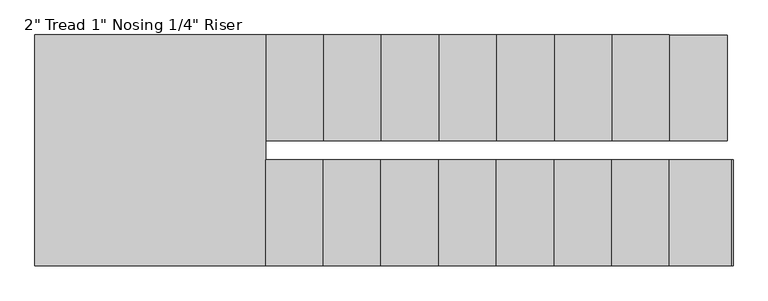
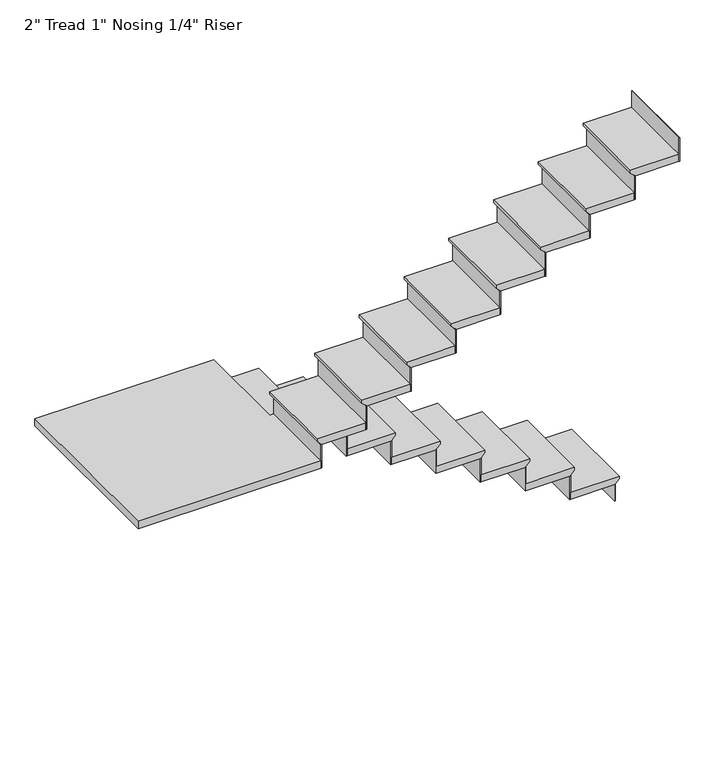
"""IFC4 building model written with IfcOpenShell, lengths in millimetres: stair flight geometry."""

from ifc_helpers import new_model, si_unit, origin, place, context, project, spatial, faceted_brep, source, transform, mapped, element, save


def stair_flight_6b4fcaec(model_context):
    return source(origin(), model_context, "Body", "Brep", [
        faceted_brep([(-1805.9198569, -5306.3933037, 12951.8833333), (-1805.9198569, -5306.3933037, 12970.9333333), (-1805.9198569, -5865.1933037, 12970.9333333), (-1805.9198569, -5865.1933037, 12951.8833333), (-1831.3198569, -5306.3933037, 12926.4833333), (-1831.3198569, -5865.1933037, 12926.4833333), (-2136.1198569, -5306.3933037, 12970.9333333), (-2136.1198569, -5865.1933037, 12970.9333333), (-1831.3198569, -5865.1933037, 12920.1333333), (-2136.1198569, -5865.1933037, 12920.1333333), (-2136.1198569, -5306.3933037, 12920.1333333), (-1831.3198569, -5306.3933037, 12920.1333333)], [[[0, 1, 2, 3]], [[4, 0, 3, 5]], [[2, 1, 6, 7]], [[8, 9, 10, 11]], [[2, 7, 9, 8, 5, 3]], [[8, 11, 4, 5]], [[6, 1, 0, 4, 11, 10]], [[7, 6, 10, 9]]]),
        faceted_brep([(-1831.3198569, -5306.3933037, 12920.1333333), (-1831.3198569, -5306.3933037, 12801.6), (-1837.6698569, -5306.3933037, 12801.6), (-1837.6698569, -5306.3933037, 12920.1333333), (-1831.3198569, -5865.1933037, 12920.1333333), (-1837.6698569, -5865.1933037, 12920.1333333), (-1837.6698569, -5865.1933037, 12801.6), (-1831.3198569, -5865.1933037, 12801.6)], [[[0, 1, 2, 3]], [[4, 5, 6, 7]], [[1, 0, 4, 7]], [[2, 1, 7, 6]], [[3, 2, 6, 5]], [[0, 3, 5, 4]]]),
        faceted_brep([(-2136.1198569, -5306.3933037, 13089.4666667), (-2136.1198569, -5306.3933037, 12920.1333333), (-2142.4698569, -5306.3933037, 12920.1333333), (-2142.4698569, -5306.3933037, 13089.4666667), (-2136.1198569, -5865.1933037, 13089.4666667), (-2142.4698569, -5865.1933037, 13089.4666667), (-2142.4698569, -5865.1933037, 12920.1333333), (-2136.1198569, -5865.1933037, 12920.1333333)], [[[0, 1, 2, 3]], [[4, 5, 6, 7]], [[1, 0, 4, 7]], [[2, 1, 7, 6]], [[3, 2, 6, 5]], [[0, 3, 5, 4]]]),
        faceted_brep([(-2110.7198569, -5865.1933037, 13140.2666667), (-2110.7198569, -5306.3933037, 13140.2666667), (-2440.9198569, -5306.3933037, 13140.2666667), (-2440.9198569, -5865.1933037, 13140.2666667), (-2136.1198569, -5865.1933037, 13089.4666667), (-2440.9198569, -5865.1933037, 13089.4666667), (-2440.9198569, -5306.3933037, 13089.4666667), (-2136.1198569, -5306.3933037, 13089.4666667), (-2136.1198569, -5865.1933037, 13095.8166667), (-2110.7198569, -5865.1933037, 13121.2166667), (-2136.1198569, -5306.3933037, 13095.8166667), (-2110.7198569, -5306.3933037, 13121.2166667)], [[[0, 1, 2, 3]], [[4, 5, 6, 7]], [[0, 3, 5, 4, 8, 9]], [[4, 7, 10, 8]], [[2, 1, 11, 10, 7, 6]], [[3, 2, 6, 5]], [[11, 1, 0, 9]], [[10, 11, 9, 8]]]),
        faceted_brep([(-2440.9198569, -5306.3933037, 13258.8), (-2440.9198569, -5306.3933037, 13089.4666667), (-2447.2698569, -5306.3933037, 13089.4666667), (-2447.2698569, -5306.3933037, 13258.8), (-2440.9198569, -5865.1933037, 13258.8), (-2447.2698569, -5865.1933037, 13258.8), (-2447.2698569, -5865.1933037, 13089.4666667), (-2440.9198569, -5865.1933037, 13089.4666667)], [[[0, 1, 2, 3]], [[4, 5, 6, 7]], [[1, 0, 4, 7]], [[2, 1, 7, 6]], [[3, 2, 6, 5]], [[0, 3, 5, 4]]]),
        faceted_brep([(-2415.5198569, -5865.1933037, 13309.6), (-2415.5198569, -5306.3933037, 13309.6), (-2745.7198569, -5306.3933037, 13309.6), (-2745.7198569, -5865.1933037, 13309.6), (-2440.9198569, -5865.1933037, 13258.8), (-2745.7198569, -5865.1933037, 13258.8), (-2745.7198569, -5306.3933037, 13258.8), (-2440.9198569, -5306.3933037, 13258.8), (-2440.9198569, -5865.1933037, 13265.15), (-2415.5198569, -5865.1933037, 13290.55), (-2440.9198569, -5306.3933037, 13265.15), (-2415.5198569, -5306.3933037, 13290.55)], [[[0, 1, 2, 3]], [[4, 5, 6, 7]], [[0, 3, 5, 4, 8, 9]], [[4, 7, 10, 8]], [[2, 1, 11, 10, 7, 6]], [[3, 2, 6, 5]], [[11, 1, 0, 9]], [[10, 11, 9, 8]]]),
        faceted_brep([(-2745.7198569, -5306.3933037, 13428.1333333), (-2745.7198569, -5306.3933037, 13258.8), (-2752.0698569, -5306.3933037, 13258.8), (-2752.0698569, -5306.3933037, 13428.1333333), (-2745.7198569, -5865.1933037, 13428.1333333), (-2752.0698569, -5865.1933037, 13428.1333333), (-2752.0698569, -5865.1933037, 13258.8), (-2745.7198569, -5865.1933037, 13258.8)], [[[0, 1, 2, 3]], [[4, 5, 6, 7]], [[1, 0, 4, 7]], [[2, 1, 7, 6]], [[3, 2, 6, 5]], [[0, 3, 5, 4]]]),
        faceted_brep([(-2720.3198569, -5865.1933037, 13478.9333333), (-2720.3198569, -5306.3933037, 13478.9333333), (-3050.5198569, -5306.3933037, 13478.9333333), (-3050.5198569, -5865.1933037, 13478.9333333), (-2745.7198569, -5865.1933037, 13428.1333333), (-3050.5198569, -5865.1933037, 13428.1333333), (-3050.5198569, -5306.3933037, 13428.1333333), (-2745.7198569, -5306.3933037, 13428.1333333), (-2745.7198569, -5865.1933037, 13434.4833333), (-2720.3198569, -5865.1933037, 13459.8833333), (-2745.7198569, -5306.3933037, 13434.4833333), (-2720.3198569, -5306.3933037, 13459.8833333)], [[[0, 1, 2, 3]], [[4, 5, 6, 7]], [[0, 3, 5, 4, 8, 9]], [[4, 7, 10, 8]], [[2, 1, 11, 10, 7, 6]], [[3, 2, 6, 5]], [[11, 1, 0, 9]], [[10, 11, 9, 8]]]),
        faceted_brep([(-3050.5198569, -5306.3933037, 13597.4666667), (-3050.5198569, -5306.3933037, 13428.1333333), (-3056.8698569, -5306.3933037, 13428.1333333), (-3056.8698569, -5306.3933037, 13597.4666667), (-3050.5198569, -5865.1933037, 13597.4666667), (-3056.8698569, -5865.1933037, 13597.4666667), (-3056.8698569, -5865.1933037, 13428.1333333), (-3050.5198569, -5865.1933037, 13428.1333333)], [[[0, 1, 2, 3]], [[4, 5, 6, 7]], [[1, 0, 4, 7]], [[2, 1, 7, 6]], [[3, 2, 6, 5]], [[0, 3, 5, 4]]]),
        faceted_brep([(-3025.1198569, -5865.1933037, 13648.2666667), (-3025.1198569, -5306.3933037, 13648.2666667), (-3355.3198569, -5306.3933037, 13648.2666667), (-3355.3198569, -5865.1933037, 13648.2666667), (-3050.5198569, -5865.1933037, 13597.4666667), (-3355.3198569, -5865.1933037, 13597.4666667), (-3355.3198569, -5306.3933037, 13597.4666667), (-3050.5198569, -5306.3933037, 13597.4666667), (-3050.5198569, -5865.1933037, 13603.8166667), (-3025.1198569, -5865.1933037, 13629.2166667), (-3050.5198569, -5306.3933037, 13603.8166667), (-3025.1198569, -5306.3933037, 13629.2166667)], [[[0, 1, 2, 3]], [[4, 5, 6, 7]], [[0, 3, 5, 4, 8, 9]], [[4, 7, 10, 8]], [[2, 1, 11, 10, 7, 6]], [[3, 2, 6, 5]], [[11, 1, 0, 9]], [[10, 11, 9, 8]]]),
        faceted_brep([(-3355.3198569, -5306.3933037, 13766.8), (-3355.3198569, -5306.3933037, 13597.4666667), (-3361.6698569, -5306.3933037, 13597.4666667), (-3361.6698569, -5306.3933037, 13766.8), (-3355.3198569, -5865.1933037, 13766.8), (-3361.6698569, -5865.1933037, 13766.8), (-3361.6698569, -5865.1933037, 13597.4666667), (-3355.3198569, -5865.1933037, 13597.4666667)], [[[0, 1, 2, 3]], [[4, 5, 6, 7]], [[1, 0, 4, 7]], [[2, 1, 7, 6]], [[3, 2, 6, 5]], [[0, 3, 5, 4]]]),
        faceted_brep([(-3329.9198569, -5865.1933037, 13817.6), (-3329.9198569, -5306.3933037, 13817.6), (-3660.1198569, -5306.3933037, 13817.6), (-3660.1198569, -5865.1933037, 13817.6), (-3355.3198569, -5865.1933037, 13766.8), (-3660.1198569, -5865.1933037, 13766.8), (-3660.1198569, -5306.3933037, 13766.8), (-3355.3198569, -5306.3933037, 13766.8), (-3355.3198569, -5865.1933037, 13773.15), (-3329.9198569, -5865.1933037, 13798.55), (-3355.3198569, -5306.3933037, 13773.15), (-3329.9198569, -5306.3933037, 13798.55)], [[[0, 1, 2, 3]], [[4, 5, 6, 7]], [[0, 3, 5, 4, 8, 9]], [[4, 7, 10, 8]], [[2, 1, 11, 10, 7, 6]], [[3, 2, 6, 5]], [[11, 1, 0, 9]], [[10, 11, 9, 8]]]),
        faceted_brep([(-3660.1198569, -5306.3933037, 13936.1333333), (-3660.1198569, -5306.3933037, 13766.8), (-3666.4698569, -5306.3933037, 13766.8), (-3666.4698569, -5306.3933037, 13936.1333333), (-3660.1198569, -5865.1933037, 13936.1333333), (-3666.4698569, -5865.1933037, 13936.1333333), (-3666.4698569, -5865.1933037, 13766.8), (-3660.1198569, -5865.1933037, 13766.8)], [[[0, 1, 2, 3]], [[4, 5, 6, 7]], [[1, 0, 4, 7]], [[2, 1, 7, 6]], [[3, 2, 6, 5]], [[0, 3, 5, 4]]]),
        faceted_brep([(-3634.7198569, -5865.1933037, 13986.9333333), (-3634.7198569, -5306.3933037, 13986.9333333), (-3964.9198569, -5306.3933037, 13986.9333333), (-3964.9198569, -5865.1933037, 13986.9333333), (-3660.1198569, -5865.1933037, 13936.1333333), (-3964.9198569, -5865.1933037, 13936.1333333), (-3964.9198569, -5306.3933037, 13936.1333333), (-3660.1198569, -5306.3933037, 13936.1333333), (-3660.1198569, -5865.1933037, 13942.4833333), (-3634.7198569, -5865.1933037, 13967.8833333), (-3660.1198569, -5306.3933037, 13942.4833333), (-3634.7198569, -5306.3933037, 13967.8833333)], [[[0, 1, 2, 3]], [[4, 5, 6, 7]], [[0, 3, 5, 4, 8, 9]], [[4, 7, 10, 8]], [[2, 1, 11, 10, 7, 6]], [[3, 2, 6, 5]], [[11, 1, 0, 9]], [[10, 11, 9, 8]]]),
        faceted_brep([(-3964.9198569, -5306.3933037, 14105.4666667), (-3964.9198569, -5306.3933037, 13936.1333333), (-3971.2698569, -5306.3933037, 13936.1333333), (-3971.2698569, -5306.3933037, 14105.4666667), (-3964.9198569, -5865.1933037, 14105.4666667), (-3971.2698569, -5865.1933037, 14105.4666667), (-3971.2698569, -5865.1933037, 13936.1333333), (-3964.9198569, -5865.1933037, 13936.1333333)], [[[0, 1, 2, 3]], [[4, 5, 6, 7]], [[1, 0, 4, 7]], [[2, 1, 7, 6]], [[3, 2, 6, 5]], [[0, 3, 5, 4]]]),
        faceted_brep([(-3939.5198569, -5865.1933037, 14156.2666667), (-3939.5198569, -5306.3933037, 14156.2666667), (-4269.7198569, -5306.3933037, 14156.2666667), (-4269.7198569, -5865.1933037, 14156.2666667), (-3964.9198569, -5865.1933037, 14105.4666667), (-4269.7198569, -5865.1933037, 14105.4666667), (-4269.7198569, -5306.3933037, 14105.4666667), (-3964.9198569, -5306.3933037, 14105.4666667), (-3964.9198569, -5865.1933037, 14111.8166667), (-3939.5198569, -5865.1933037, 14137.2166667), (-3964.9198569, -5306.3933037, 14111.8166667), (-3939.5198569, -5306.3933037, 14137.2166667)], [[[0, 1, 2, 3]], [[4, 5, 6, 7]], [[0, 3, 5, 4, 8, 9]], [[4, 7, 10, 8]], [[2, 1, 11, 10, 7, 6]], [[3, 2, 6, 5]], [[11, 1, 0, 9]], [[10, 11, 9, 8]]]),
        faceted_brep([(-4269.7198569, -5306.3933037, 14274.8), (-4269.7198569, -5306.3933037, 14105.4666667), (-4276.0698569, -5306.3933037, 14105.4666667), (-4276.0698569, -5306.3933037, 14274.8), (-4269.7198569, -5865.1933037, 14274.8), (-4276.0698569, -5865.1933037, 14274.8), (-4276.0698569, -5865.1933037, 14105.4666667), (-4269.7198569, -5865.1933037, 14105.4666667)], [[[0, 1, 2, 3]], [[4, 5, 6, 7]], [[1, 0, 4, 7]], [[2, 1, 7, 6]], [[3, 2, 6, 5]], [[0, 3, 5, 4]]]),
        faceted_brep([(-4218.9198569, -5966.7933037, 14325.6), (-4244.3198569, -5966.7933037, 14325.6), (-4244.3198569, -5306.3933037, 14325.6), (-5463.5198569, -5306.3933037, 14325.6), (-5463.5198569, -6525.5933037, 14325.6), (-4218.9198569, -6525.5933037, 14325.6), (-4244.3198569, -5966.7933037, 14274.8), (-4218.9198569, -5966.7933037, 14274.8), (-4218.9198569, -6525.5933037, 14274.8), (-5463.5198569, -6525.5933037, 14274.8), (-5463.5198569, -5306.3933037, 14274.8), (-4269.7198569, -5306.3933037, 14274.8), (-4269.7198569, -5865.1933037, 14274.8), (-4244.3198569, -5865.1933037, 14274.8), (-4244.3198569, -5865.1933037, 14306.55), (-4244.3198569, -5306.3933037, 14306.55), (-4269.7198569, -5865.1933037, 14281.15), (-4269.7198569, -5306.3933037, 14281.15)], [[[0, 1, 2, 3, 4, 5]], [[6, 7, 8, 9, 10, 11, 12, 13]], [[1, 0, 7, 6]], [[2, 1, 6, 13, 14, 15]], [[13, 12, 16, 14]], [[12, 11, 17, 16]], [[3, 2, 15, 17, 11, 10]], [[4, 3, 10, 9]], [[5, 4, 9, 8]], [[0, 5, 8, 7]], [[17, 15, 14, 16]]]),
        faceted_brep([(-4218.9198569, -6525.5933037, 14444.1333333), (-4218.9198569, -6525.5933037, 14274.8), (-4212.5698569, -6525.5933037, 14274.8), (-4212.5698569, -6525.5933037, 14444.1333333), (-4218.9198569, -5966.7933037, 14444.1333333), (-4212.5698569, -5966.7933037, 14444.1333333), (-4212.5698569, -5966.7933037, 14274.8), (-4218.9198569, -5966.7933037, 14274.8)], [[[0, 1, 2, 3]], [[4, 5, 6, 7]], [[1, 0, 4, 7]], [[2, 1, 7, 6]], [[3, 2, 6, 5]], [[0, 3, 5, 4]]]),
        faceted_brep([(-4244.3198569, -5966.7933037, 14494.9333333), (-4244.3198569, -6525.5933037, 14494.9333333), (-3914.1198569, -6525.5933037, 14494.9333333), (-3914.1198569, -5966.7933037, 14494.9333333), (-4218.9198569, -5966.7933037, 14444.1333333), (-3914.1198569, -5966.7933037, 14444.1333333), (-3914.1198569, -6525.5933037, 14444.1333333), (-4218.9198569, -6525.5933037, 14444.1333333), (-4218.9198569, -5966.7933037, 14450.4833333), (-4244.3198569, -5966.7933037, 14475.8833333), (-4218.9198569, -6525.5933037, 14450.4833333), (-4244.3198569, -6525.5933037, 14475.8833333)], [[[0, 1, 2, 3]], [[4, 5, 6, 7]], [[0, 3, 5, 4, 8, 9]], [[4, 7, 10, 8]], [[2, 1, 11, 10, 7, 6]], [[3, 2, 6, 5]], [[11, 1, 0, 9]], [[10, 11, 9, 8]]]),
        faceted_brep([(-3914.1198569, -6525.5933037, 14613.4666667), (-3914.1198569, -6525.5933037, 14444.1333333), (-3907.7698569, -6525.5933037, 14444.1333333), (-3907.7698569, -6525.5933037, 14613.4666667), (-3914.1198569, -5966.7933037, 14613.4666667), (-3907.7698569, -5966.7933037, 14613.4666667), (-3907.7698569, -5966.7933037, 14444.1333333), (-3914.1198569, -5966.7933037, 14444.1333333)], [[[0, 1, 2, 3]], [[4, 5, 6, 7]], [[1, 0, 4, 7]], [[2, 1, 7, 6]], [[3, 2, 6, 5]], [[0, 3, 5, 4]]]),
        faceted_brep([(-3939.5198569, -5966.7933037, 14664.2666667), (-3939.5198569, -6525.5933037, 14664.2666667), (-3609.3198569, -6525.5933037, 14664.2666667), (-3609.3198569, -5966.7933037, 14664.2666667), (-3914.1198569, -5966.7933037, 14613.4666667), (-3609.3198569, -5966.7933037, 14613.4666667), (-3609.3198569, -6525.5933037, 14613.4666667), (-3914.1198569, -6525.5933037, 14613.4666667), (-3914.1198569, -5966.7933037, 14619.8166667), (-3939.5198569, -5966.7933037, 14645.2166667), (-3914.1198569, -6525.5933037, 14619.8166667), (-3939.5198569, -6525.5933037, 14645.2166667)], [[[0, 1, 2, 3]], [[4, 5, 6, 7]], [[0, 3, 5, 4, 8, 9]], [[4, 7, 10, 8]], [[2, 1, 11, 10, 7, 6]], [[3, 2, 6, 5]], [[11, 1, 0, 9]], [[10, 11, 9, 8]]]),
        faceted_brep([(-3609.3198569, -6525.5933037, 14782.8), (-3609.3198569, -6525.5933037, 14613.4666667), (-3602.9698569, -6525.5933037, 14613.4666667), (-3602.9698569, -6525.5933037, 14782.8), (-3609.3198569, -5966.7933037, 14782.8), (-3602.9698569, -5966.7933037, 14782.8), (-3602.9698569, -5966.7933037, 14613.4666667), (-3609.3198569, -5966.7933037, 14613.4666667)], [[[0, 1, 2, 3]], [[4, 5, 6, 7]], [[1, 0, 4, 7]], [[2, 1, 7, 6]], [[3, 2, 6, 5]], [[0, 3, 5, 4]]]),
        faceted_brep([(-3634.7198569, -5966.7933037, 14833.6), (-3634.7198569, -6525.5933037, 14833.6), (-3304.5198569, -6525.5933037, 14833.6), (-3304.5198569, -5966.7933037, 14833.6), (-3609.3198569, -5966.7933037, 14782.8), (-3304.5198569, -5966.7933037, 14782.8), (-3304.5198569, -6525.5933037, 14782.8), (-3609.3198569, -6525.5933037, 14782.8), (-3609.3198569, -5966.7933037, 14789.15), (-3634.7198569, -5966.7933037, 14814.55), (-3609.3198569, -6525.5933037, 14789.15), (-3634.7198569, -6525.5933037, 14814.55)], [[[0, 1, 2, 3]], [[4, 5, 6, 7]], [[0, 3, 5, 4, 8, 9]], [[4, 7, 10, 8]], [[2, 1, 11, 10, 7, 6]], [[3, 2, 6, 5]], [[11, 1, 0, 9]], [[10, 11, 9, 8]]]),
        faceted_brep([(-3304.5198569, -6525.5933037, 14952.1333333), (-3304.5198569, -6525.5933037, 14782.8), (-3298.1698569, -6525.5933037, 14782.8), (-3298.1698569, -6525.5933037, 14952.1333333), (-3304.5198569, -5966.7933037, 14952.1333333), (-3298.1698569, -5966.7933037, 14952.1333333), (-3298.1698569, -5966.7933037, 14782.8), (-3304.5198569, -5966.7933037, 14782.8)], [[[0, 1, 2, 3]], [[4, 5, 6, 7]], [[1, 0, 4, 7]], [[2, 1, 7, 6]], [[3, 2, 6, 5]], [[0, 3, 5, 4]]]),
        faceted_brep([(-3329.9198569, -5966.7933037, 15002.9333333), (-3329.9198569, -6525.5933037, 15002.9333333), (-2999.7198569, -6525.5933037, 15002.9333333), (-2999.7198569, -5966.7933037, 15002.9333333), (-3304.5198569, -5966.7933037, 14952.1333333), (-2999.7198569, -5966.7933037, 14952.1333333), (-2999.7198569, -6525.5933037, 14952.1333333), (-3304.5198569, -6525.5933037, 14952.1333333), (-3304.5198569, -5966.7933037, 14958.4833333), (-3329.9198569, -5966.7933037, 14983.8833333), (-3304.5198569, -6525.5933037, 14958.4833333), (-3329.9198569, -6525.5933037, 14983.8833333)], [[[0, 1, 2, 3]], [[4, 5, 6, 7]], [[0, 3, 5, 4, 8, 9]], [[4, 7, 10, 8]], [[2, 1, 11, 10, 7, 6]], [[3, 2, 6, 5]], [[11, 1, 0, 9]], [[10, 11, 9, 8]]]),
        faceted_brep([(-2999.7198569, -6525.5933037, 15121.4666667), (-2999.7198569, -6525.5933037, 14952.1333333), (-2993.3698569, -6525.5933037, 14952.1333333), (-2993.3698569, -6525.5933037, 15121.4666667), (-2999.7198569, -5966.7933037, 15121.4666667), (-2993.3698569, -5966.7933037, 15121.4666667), (-2993.3698569, -5966.7933037, 14952.1333333), (-2999.7198569, -5966.7933037, 14952.1333333)], [[[0, 1, 2, 3]], [[4, 5, 6, 7]], [[1, 0, 4, 7]], [[2, 1, 7, 6]], [[3, 2, 6, 5]], [[0, 3, 5, 4]]]),
        faceted_brep([(-3025.1198569, -5966.7933037, 15172.2666667), (-3025.1198569, -6525.5933037, 15172.2666667), (-2694.9198569, -6525.5933037, 15172.2666667), (-2694.9198569, -5966.7933037, 15172.2666667), (-2999.7198569, -5966.7933037, 15121.4666667), (-2694.9198569, -5966.7933037, 15121.4666667), (-2694.9198569, -6525.5933037, 15121.4666667), (-2999.7198569, -6525.5933037, 15121.4666667), (-2999.7198569, -5966.7933037, 15127.8166667), (-3025.1198569, -5966.7933037, 15153.2166667), (-2999.7198569, -6525.5933037, 15127.8166667), (-3025.1198569, -6525.5933037, 15153.2166667)], [[[0, 1, 2, 3]], [[4, 5, 6, 7]], [[0, 3, 5, 4, 8, 9]], [[4, 7, 10, 8]], [[2, 1, 11, 10, 7, 6]], [[3, 2, 6, 5]], [[11, 1, 0, 9]], [[10, 11, 9, 8]]]),
        faceted_brep([(-2694.9198569, -6525.5933037, 15290.8), (-2694.9198569, -6525.5933037, 15121.4666667), (-2688.5698569, -6525.5933037, 15121.4666667), (-2688.5698569, -6525.5933037, 15290.8), (-2694.9198569, -5966.7933037, 15290.8), (-2688.5698569, -5966.7933037, 15290.8), (-2688.5698569, -5966.7933037, 15121.4666667), (-2694.9198569, -5966.7933037, 15121.4666667)], [[[0, 1, 2, 3]], [[4, 5, 6, 7]], [[1, 0, 4, 7]], [[2, 1, 7, 6]], [[3, 2, 6, 5]], [[0, 3, 5, 4]]]),
        faceted_brep([(-2720.3198569, -5966.7933037, 15341.6), (-2720.3198569, -6525.5933037, 15341.6), (-2390.1198569, -6525.5933037, 15341.6), (-2390.1198569, -5966.7933037, 15341.6), (-2694.9198569, -5966.7933037, 15290.8), (-2390.1198569, -5966.7933037, 15290.8), (-2390.1198569, -6525.5933037, 15290.8), (-2694.9198569, -6525.5933037, 15290.8), (-2694.9198569, -5966.7933037, 15297.15), (-2720.3198569, -5966.7933037, 15322.55), (-2694.9198569, -6525.5933037, 15297.15), (-2720.3198569, -6525.5933037, 15322.55)], [[[0, 1, 2, 3]], [[4, 5, 6, 7]], [[0, 3, 5, 4, 8, 9]], [[4, 7, 10, 8]], [[2, 1, 11, 10, 7, 6]], [[3, 2, 6, 5]], [[11, 1, 0, 9]], [[10, 11, 9, 8]]]),
        faceted_brep([(-2390.1198569, -6525.5933037, 15460.1333333), (-2390.1198569, -6525.5933037, 15290.8), (-2383.7698569, -6525.5933037, 15290.8), (-2383.7698569, -6525.5933037, 15460.1333333), (-2390.1198569, -5966.7933037, 15460.1333333), (-2383.7698569, -5966.7933037, 15460.1333333), (-2383.7698569, -5966.7933037, 15290.8), (-2390.1198569, -5966.7933037, 15290.8)], [[[0, 1, 2, 3]], [[4, 5, 6, 7]], [[1, 0, 4, 7]], [[2, 1, 7, 6]], [[3, 2, 6, 5]], [[0, 3, 5, 4]]]),
        faceted_brep([(-2415.5198569, -5966.7933037, 15510.9333333), (-2415.5198569, -6525.5933037, 15510.9333333), (-2085.3198569, -6525.5933037, 15510.9333333), (-2085.3198569, -5966.7933037, 15510.9333333), (-2390.1198569, -5966.7933037, 15460.1333333), (-2085.3198569, -5966.7933037, 15460.1333333), (-2085.3198569, -6525.5933037, 15460.1333333), (-2390.1198569, -6525.5933037, 15460.1333333), (-2390.1198569, -5966.7933037, 15466.4833333), (-2415.5198569, -5966.7933037, 15491.8833333), (-2390.1198569, -6525.5933037, 15466.4833333), (-2415.5198569, -6525.5933037, 15491.8833333)], [[[0, 1, 2, 3]], [[4, 5, 6, 7]], [[0, 3, 5, 4, 8, 9]], [[4, 7, 10, 8]], [[2, 1, 11, 10, 7, 6]], [[3, 2, 6, 5]], [[11, 1, 0, 9]], [[10, 11, 9, 8]]]),
        faceted_brep([(-2085.3198569, -6525.5933037, 15629.4666667), (-2085.3198569, -6525.5933037, 15460.1333333), (-2078.9698569, -6525.5933037, 15460.1333333), (-2078.9698569, -6525.5933037, 15629.4666667), (-2085.3198569, -5966.7933037, 15629.4666667), (-2078.9698569, -5966.7933037, 15629.4666667), (-2078.9698569, -5966.7933037, 15460.1333333), (-2085.3198569, -5966.7933037, 15460.1333333)], [[[0, 1, 2, 3]], [[4, 5, 6, 7]], [[1, 0, 4, 7]], [[2, 1, 7, 6]], [[3, 2, 6, 5]], [[0, 3, 5, 4]]]),
        faceted_brep([(-1780.5198569, -6525.5933037, 15798.8), (-1780.5198569, -6525.5933037, 15629.4666667), (-1774.1698569, -6525.5933037, 15629.4666667), (-1774.1698569, -6525.5933037, 15798.8), (-1780.5198569, -5966.7933037, 15798.8), (-1774.1698569, -5966.7933037, 15798.8), (-1774.1698569, -5966.7933037, 15629.4666667), (-1780.5198569, -5966.7933037, 15629.4666667)], [[[0, 1, 2, 3]], [[4, 5, 6, 7]], [[1, 0, 4, 7]], [[2, 1, 7, 6]], [[3, 2, 6, 5]], [[0, 3, 5, 4]]]),
        faceted_brep([(-2110.7198569, -5966.7933037, 15680.2666667), (-2110.7198569, -6525.5933037, 15680.2666667), (-1780.5198569, -6525.5933037, 15680.2666667), (-1780.5198569, -5966.7933037, 15680.2666667), (-2085.3198569, -5966.7933037, 15629.4666667), (-1780.5198569, -5966.7933037, 15629.4666667), (-1780.5198569, -6525.5933037, 15629.4666667), (-2085.3198569, -6525.5933037, 15629.4666667), (-2085.3198569, -5966.7933037, 15635.8166667), (-2110.7198569, -5966.7933037, 15661.2166667), (-2085.3198569, -6525.5933037, 15635.8166667), (-2110.7198569, -6525.5933037, 15661.2166667)], [[[0, 1, 2, 3]], [[4, 5, 6, 7]], [[0, 3, 5, 4, 8, 9]], [[4, 7, 10, 8]], [[2, 1, 11, 10, 7, 6]], [[3, 2, 6, 5]], [[11, 1, 0, 9]], [[10, 11, 9, 8]]]),
    ])


if __name__ == "__main__":
    model = new_model("IFC4")
    model_context = context("Model", 3, world=origin())
    ifc_project = project(units=[si_unit("LENGTHUNIT", "METRE", prefix="MILLI")], contexts=[model_context])
    site = spatial("IfcSite", under=ifc_project)
    building = spatial("IfcBuilding", under=site)
    placement = place(None, origin())
    stair_flight_shape = stair_flight_6b4fcaec(model_context)
    element("IfcStairFlight", 1, ObjectType="2\" Tread 1\" Nosing 1/4\" Riser", at=placement, inside=building, context=model_context, shape_type="MappedRepresentation", body=[
        mapped(stair_flight_shape, transform((0.0, 0.0, 0.0), x_axis=(1.0, 0.0, 0.0), y_axis=(0.0, 1.0, 0.0), z_axis=(0.0, 0.0, 1.0))),
    ])
    save(model, "model.ifc")
